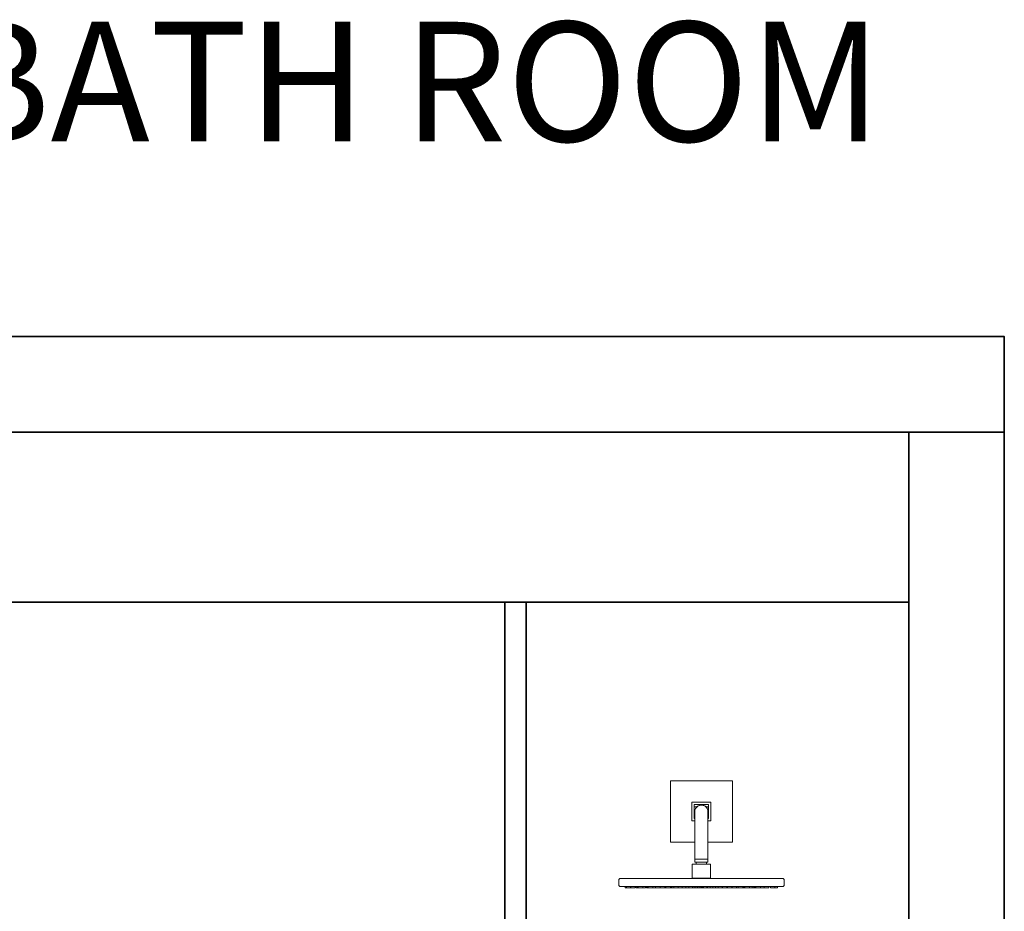
# Model space of a CAD drawing. Units: inches. Extents: x 64 to 1167, y 117 to 939.
# Tile 56 of 56: x 1074 to 1167, y 512 to 596. Entities that reach past the tile are written whole.
import ezdxf

# ---------------------------------------------------------------- set-up
doc = ezdxf.new("R2010")
doc.units = ezdxf.units.IN
doc.header["$MEASUREMENT"] = 0
for name, color, linetype, lineweight in [('A-ANNO-TEXT', 7, 'Continuous', 25), ('A-FLOR-FIXT', 8, 'Continuous', 18), ('A-SECT', 7, 'Continuous', 35)]:
    doc.layers.add(name, color=color, linetype=linetype, lineweight=lineweight)
doc.styles.get("Standard").update_dxf_attribs({"font": 'arial.ttf'})

msp = doc.modelspace()

# ---------------------------------------------------------------- linework, layer by layer
at = {"layer": 'A-FLOR-FIXT'}
for p, q in [((1141.249, 523.875), (1135.4, 523.875)), ((1135.4, 518.097), (1135.4, 523.875)), ((1141.249, 518.097), (1141.249, 523.875)), ((1137.42, 520.097), (1137.42, 521.875)), ((1137.429, 521.875), (1137.42, 521.875)), ((1137.438, 521.875), (1137.429, 521.875)), ((1137.447, 521.875), (1137.438, 521.875)), ((1137.455, 521.875), (1137.447, 521.875)), ((1137.462, 521.875), (1137.455, 521.875)), ((1137.468, 521.875), (1137.462, 521.875)), ((1137.473, 521.875), (1137.468, 521.875)), ((1137.477, 521.875), (1137.473, 521.875)), ((1137.48, 521.875), (1137.477, 521.875)), ((1137.482, 521.875), (1137.48, 521.875)), ((1137.48, 521.875), (1137.483, 521.875)), ((1139.148, 521.875), (1137.483, 521.875)), ((1139.15, 521.875), (1139.148, 521.875)), ((1139.153, 521.875), (1139.15, 521.875)), ((1139.157, 521.875), (1139.153, 521.875)), ((1139.162, 521.875), (1139.157, 521.875)), ((1139.169, 521.875), (1139.162, 521.875)), ((1139.176, 521.875), (1139.169, 521.875)), ((1139.184, 521.875), (1139.176, 521.875)), ((1139.192, 521.875), (1139.184, 521.875)), ((1139.201, 521.875), (1139.192, 521.875)), ((1139.21, 521.875), (1139.201, 521.875)), ((1139.21, 520.097), (1139.21, 521.875)), ((1137.641, 521.43), (1137.641, 521.653)), ((1137.641, 521.653), (1138.991, 521.653)), ((1137.882, 521.43), (1137.641, 521.43)), ((1137.641, 520.319), (1137.641, 521.43)), ((1137.681, 520.967), (1137.702, 521.128)), ((1137.702, 520.806), (1137.681, 520.967)), ((1137.681, 520.319), (1137.681, 520.967)), ((1137.694, 520.986), (1137.702, 521.054)), ((1137.702, 520.918), (1137.694, 520.986)), ((1137.702, 521.128), (1137.765, 521.278)), ((1137.765, 521.278), (1137.774, 521.291)), ((1137.774, 521.291), (1137.777, 521.297)), ((1137.777, 521.297), (1137.864, 521.407)), ((1137.864, 521.407), (1137.894, 521.43)), ((1137.864, 521.407), (1137.876, 521.426)), ((1137.876, 521.426), (1137.882, 521.43)), ((1137.882, 521.43), (1138.005, 521.525)), ((1137.894, 521.43), (1137.882, 521.43)), ((1137.894, 521.43), (1137.992, 521.506)), ((1137.992, 521.506), (1138.142, 521.568)), ((1138.005, 521.525), (1138.155, 521.587)), ((1138.142, 521.568), (1138.303, 521.589)), ((1138.155, 521.587), (1138.316, 521.608)), ((1138.303, 521.589), (1138.464, 521.568)), ((1138.316, 521.608), (1138.477, 521.587)), ((1138.464, 521.568), (1138.615, 521.506)), ((1138.477, 521.587), (1138.627, 521.525)), ((1138.615, 521.506), (1138.713, 521.43)), ((1138.627, 521.525), (1138.75, 521.43)), ((1138.75, 521.43), (1138.713, 521.43)), ((1138.713, 521.43), (1138.743, 521.407)), ((1138.743, 521.407), (1138.842, 521.278)), ((1138.991, 521.43), (1138.75, 521.43)), ((1138.75, 521.43), (1138.756, 521.426)), ((1138.756, 521.426), (1138.855, 521.297)), ((1138.842, 521.278), (1138.904, 521.128)), ((1138.855, 521.297), (1138.917, 521.147)), ((1138.904, 521.128), (1138.926, 520.967)), ((1138.917, 521.147), (1138.938, 520.986)), ((1138.938, 520.986), (1138.926, 520.893)), ((1138.926, 520.893), (1138.926, 520.967)), ((1138.926, 520.319), (1138.926, 520.893)), ((1138.991, 521.43), (1138.991, 521.653)), ((1138.991, 520.319), (1138.991, 521.43)), ((1137.429, 520.097), (1137.42, 520.097)), ((1137.438, 520.097), (1137.429, 520.097)), ((1137.447, 520.097), (1137.438, 520.097)), ((1137.455, 520.097), (1137.447, 520.097)), ((1137.462, 520.097), (1137.455, 520.097)), ((1137.468, 520.097), (1137.462, 520.097)), ((1137.473, 520.097), (1137.468, 520.097)), ((1137.477, 520.097), (1137.473, 520.097)), ((1137.48, 520.097), (1137.477, 520.097)), ((1137.482, 520.097), (1137.48, 520.097)), ((1137.482, 520.097), (1137.483, 520.097)), ((1137.483, 520.097), (1137.681, 520.097)), ((1137.641, 520.319), (1137.681, 520.319)), ((1137.681, 520.097), (1137.681, 520.319)), ((1137.681, 518.097), (1137.681, 520.097)), ((1138.926, 520.319), (1138.991, 520.319)), ((1138.926, 520.097), (1138.926, 520.319)), ((1138.926, 520.097), (1139.148, 520.097)), ((1138.926, 518.097), (1138.926, 520.097)), ((1139.15, 520.097), (1139.148, 520.097)), ((1139.153, 520.097), (1139.15, 520.097)), ((1139.157, 520.097), (1139.153, 520.097)), ((1139.162, 520.097), (1139.157, 520.097)), ((1139.169, 520.097), (1139.162, 520.097)), ((1139.176, 520.097), (1139.169, 520.097)), ((1139.184, 520.097), (1139.176, 520.097)), ((1139.192, 520.097), (1139.184, 520.097)), ((1139.201, 520.097), (1139.192, 520.097)), ((1139.21, 520.097), (1139.201, 520.097)), ((1135.4, 518.097), (1137.681, 518.097)), ((1137.681, 518.097), (1137.702, 518.097)), ((1137.681, 516.515), (1137.681, 518.097)), ((1138.926, 518.097), (1141.249, 518.097)), ((1138.926, 516.515), (1138.926, 518.097)), ((1137.681, 516.204), (1137.681, 516.515)), ((1138.926, 516.515), (1137.681, 516.515)), ((1137.828, 516.204), (1137.681, 516.204)), ((1137.828, 516.204), (1137.828, 516.035)), ((1138.779, 516.204), (1137.828, 516.204)), ((1138.779, 516.204), (1138.779, 516.035)), ((1138.926, 516.204), (1138.779, 516.204)), ((1138.926, 516.204), (1138.926, 516.515)), ((1137.442, 516.035), (1137.442, 514.726)), ((1137.442, 516.035), (1137.828, 516.035)), ((1137.828, 516.035), (1138.779, 516.035)), ((1138.779, 516.035), (1139.165, 516.035)), ((1139.165, 516.035), (1139.165, 514.726)), ((1130.617, 514.681), (1130.528, 514.592)), ((1130.528, 514.592), (1130.528, 514.015)), ((1130.617, 514.681), (1137.668, 514.681)), ((1137.442, 514.726), (1137.668, 514.726)), ((1137.668, 514.726), (1137.668, 514.681)), ((1138.939, 514.726), (1137.668, 514.726)), ((1137.668, 514.681), (1138.939, 514.681)), ((1138.939, 514.726), (1138.939, 514.681)), ((1138.939, 514.726), (1139.165, 514.726)), ((1145.992, 514.681), (1138.939, 514.681)), ((1145.992, 514.681), (1146.081, 514.592)), ((1146.081, 514.592), (1146.081, 514.015)), ((1130.617, 513.926), (1130.528, 514.015)), ((1131.125, 513.926), (1130.617, 513.926)), ((1131.125, 513.926), (1131.125, 513.793)), ((1131.262, 513.926), (1131.125, 513.926)), ((1131.125, 513.793), (1131.262, 513.793)), ((1131.262, 513.926), (1131.262, 513.793)), ((1131.262, 513.926), (1131.622, 513.926)), ((1131.262, 513.793), (1131.622, 513.793)), ((1131.622, 513.926), (1131.632, 513.926)), ((1131.622, 513.926), (1131.622, 513.793)), ((1131.632, 513.926), (1131.674, 513.926)), ((1131.632, 513.926), (1131.632, 513.793)), ((1131.632, 513.793), (1131.674, 513.793)), ((1131.674, 513.926), (1131.674, 513.793)), ((1131.674, 513.926), (1132.079, 513.926)), ((1131.674, 513.793), (1132.079, 513.793)), ((1132.079, 513.926), (1132.079, 513.793)), ((1132.162, 513.926), (1132.079, 513.926)), ((1132.162, 513.926), (1132.279, 513.926)), ((1132.162, 513.926), (1132.162, 513.793)), ((1132.279, 513.793), (1132.162, 513.793)), ((1132.279, 513.926), (1132.279, 513.793)), ((1132.279, 513.926), (1132.357, 513.926)), ((1132.357, 513.793), (1132.279, 513.793)), ((1132.357, 513.926), (1132.357, 513.793)), ((1132.357, 513.926), (1132.791, 513.926)), ((1132.357, 513.793), (1132.791, 513.793)), ((1132.791, 513.926), (1132.791, 513.793)), ((1133.032, 513.926), (1132.791, 513.926)), ((1133.032, 513.793), (1132.791, 513.793)), ((1133.032, 513.926), (1133.154, 513.926)), ((1133.032, 513.926), (1133.032, 513.793)), ((1133.154, 513.926), (1133.199, 513.926)), ((1133.154, 513.926), (1133.154, 513.793)), ((1133.154, 513.793), (1133.199, 513.793)), ((1133.199, 513.926), (1133.209, 513.926)), ((1133.199, 513.926), (1133.199, 513.793)), ((1133.199, 513.793), (1133.209, 513.793)), ((1133.209, 513.926), (1133.285, 513.926)), ((1133.209, 513.926), (1133.209, 513.793)), ((1133.285, 513.793), (1133.209, 513.793)), ((1133.285, 513.926), (1133.285, 513.793)), ((1133.285, 513.926), (1133.729, 513.926)), ((1133.285, 513.793), (1133.729, 513.793)), ((1133.729, 513.926), (1133.986, 513.926)), ((1133.729, 513.926), (1133.729, 513.793)), ((1133.986, 513.793), (1133.729, 513.793)), ((1133.986, 513.926), (1134, 513.926)), ((1133.986, 513.926), (1133.986, 513.793)), ((1133.986, 513.793), (1134, 513.793)), ((1134, 513.926), (1134, 513.793)), ((1134, 513.926), (1134.418, 513.926)), ((1134, 513.793), (1134.418, 513.793)), ((1134.418, 513.926), (1134.418, 513.793)), ((1134.418, 513.926), (1134.855, 513.926)), ((1134.418, 513.793), (1134.855, 513.793)), ((1134.855, 513.926), (1134.855, 513.793)), ((1134.855, 513.926), (1134.968, 513.926)), ((1134.968, 513.793), (1134.855, 513.793)), ((1134.968, 513.926), (1134.968, 513.793)), ((1134.968, 513.926), (1135.405, 513.926)), ((1135.405, 513.793), (1134.968, 513.793)), ((1135.405, 513.926), (1135.431, 513.926)), ((1135.405, 513.926), (1135.405, 513.793)), ((1135.405, 513.793), (1135.431, 513.793)), ((1135.431, 513.926), (1135.517, 513.926)), ((1135.431, 513.926), (1135.431, 513.793)), ((1135.517, 513.793), (1135.431, 513.793)), ((1135.517, 513.926), (1135.711, 513.926)), ((1135.517, 513.926), (1135.517, 513.793)), ((1135.517, 513.793), (1135.711, 513.793)), ((1135.711, 513.926), (1135.711, 513.793)), ((1135.711, 513.926), (1136.123, 513.926)), ((1135.711, 513.793), (1136.123, 513.793)), ((1136.123, 513.926), (1136.123, 513.793)), ((1136.484, 513.926), (1136.123, 513.926)), ((1136.123, 513.793), (1136.484, 513.793)), ((1136.484, 513.926), (1136.484, 513.793)), ((1136.484, 513.926), (1136.845, 513.926)), ((1136.484, 513.793), (1136.618, 513.793)), ((1136.616, 513.793), (1136.618, 513.793)), ((1136.845, 513.793), (1136.618, 513.793)), ((1136.845, 513.926), (1136.845, 513.793)), ((1136.845, 513.926), (1137.11, 513.926)), ((1137.11, 513.793), (1136.845, 513.793)), ((1137.11, 513.926), (1137.11, 513.793)), ((1137.48, 513.926), (1137.11, 513.926)), ((1137.11, 513.793), (1137.48, 513.793)), ((1137.48, 513.926), (1137.48, 513.793)), ((1137.48, 513.926), (1137.638, 513.926)), ((1137.48, 513.793), (1137.638, 513.793)), ((1137.638, 513.926), (1137.638, 513.793)), ((1137.638, 513.926), (1137.795, 513.926)), ((1137.795, 513.793), (1137.638, 513.793)), ((1137.795, 513.926), (1137.795, 513.793)), ((1137.795, 513.926), (1137.953, 513.926)), ((1137.953, 513.793), (1137.795, 513.793)), ((1137.953, 513.926), (1137.953, 513.793)), ((1137.953, 513.926), (1138.111, 513.926)), ((1138.111, 513.793), (1137.953, 513.793)), ((1138.111, 513.926), (1138.111, 513.793)), ((1138.269, 513.926), (1138.111, 513.926)), ((1138.269, 513.793), (1138.111, 513.793)), ((1138.269, 513.926), (1138.285, 513.926)), ((1138.269, 513.926), (1138.269, 513.793)), ((1138.269, 513.793), (1138.285, 513.793)), ((1138.285, 513.926), (1138.331, 513.926)), ((1138.285, 513.926), (1138.285, 513.793)), ((1138.285, 513.793), (1138.331, 513.793)), ((1138.331, 513.926), (1138.376, 513.926)), ((1138.331, 513.926), (1138.331, 513.793)), ((1138.376, 513.793), (1138.331, 513.793)), ((1138.376, 513.926), (1138.421, 513.926)), ((1138.376, 513.926), (1138.376, 513.793)), ((1138.421, 513.793), (1138.376, 513.793)), ((1138.421, 513.926), (1138.466, 513.926)), ((1138.421, 513.926), (1138.421, 513.793)), ((1138.466, 513.793), (1138.421, 513.793)), ((1138.466, 513.926), (1138.512, 513.926)), ((1138.466, 513.926), (1138.466, 513.793)), ((1138.466, 513.793), (1138.512, 513.793)), ((1138.512, 513.926), (1138.826, 513.926)), ((1138.512, 513.926), (1138.512, 513.793)), ((1138.826, 513.793), (1138.512, 513.793)), ((1138.826, 513.926), (1138.826, 513.793)), ((1138.826, 513.926), (1138.875, 513.926)), ((1138.875, 513.793), (1138.826, 513.793)), ((1138.875, 513.926), (1138.875, 513.793)), ((1139.128, 513.926), (1138.875, 513.926)), ((1138.875, 513.793), (1139.128, 513.793)), ((1139.128, 513.926), (1139.128, 513.793)), ((1139.128, 513.926), (1139.381, 513.926)), ((1139.381, 513.793), (1139.128, 513.793)), ((1139.381, 513.926), (1139.381, 513.793)), ((1139.634, 513.926), (1139.381, 513.926)), ((1139.634, 513.793), (1139.381, 513.793)), ((1139.634, 513.926), (1139.634, 513.793)), ((1139.887, 513.926), (1139.634, 513.926)), ((1139.634, 513.793), (1139.887, 513.793)), ((1139.887, 513.926), (1139.887, 513.793)), ((1139.887, 513.926), (1140.258, 513.926)), ((1140.258, 513.793), (1139.887, 513.793)), ((1140.258, 513.926), (1140.258, 513.793)), ((1140.258, 513.926), (1140.297, 513.926)), ((1140.258, 513.793), (1140.297, 513.793)), ((1140.297, 513.926), (1140.297, 513.793)), ((1140.71, 513.926), (1140.297, 513.926)), ((1140.71, 513.793), (1140.297, 513.793)), ((1140.71, 513.926), (1140.71, 513.793)), ((1140.71, 513.926), (1140.748, 513.926)), ((1140.71, 513.793), (1140.748, 513.793)), ((1140.748, 513.926), (1140.748, 513.793)), ((1140.748, 513.926), (1141.16, 513.926)), ((1141.16, 513.793), (1140.748, 513.793)), ((1141.16, 513.926), (1141.16, 513.793)), ((1141.16, 513.926), (1141.198, 513.926)), ((1141.16, 513.793), (1141.198, 513.793)), ((1141.198, 513.926), (1141.198, 513.793)), ((1141.611, 513.926), (1141.198, 513.926)), ((1141.611, 513.793), (1141.198, 513.793)), ((1141.611, 513.926), (1141.611, 513.793)), ((1141.611, 513.926), (1141.761, 513.926)), ((1141.761, 513.793), (1141.611, 513.793)), ((1141.761, 513.926), (1141.761, 513.793)), ((1141.761, 513.926), (1142.198, 513.926)), ((1142.198, 513.793), (1141.761, 513.793)), ((1142.198, 513.926), (1142.198, 513.793)), ((1142.198, 513.926), (1142.294, 513.926)), ((1142.294, 513.793), (1142.198, 513.793)), ((1142.294, 513.926), (1142.294, 513.793)), ((1142.371, 513.926), (1142.294, 513.926)), ((1142.371, 513.793), (1142.294, 513.793)), ((1142.371, 513.926), (1142.371, 513.793)), ((1142.371, 513.926), (1142.39, 513.926)), ((1142.371, 513.793), (1142.39, 513.793)), ((1142.39, 513.926), (1142.39, 513.793)), ((1142.828, 513.926), (1142.39, 513.926)), ((1142.828, 513.793), (1142.39, 513.793)), ((1142.828, 513.926), (1142.828, 513.793)), ((1142.828, 513.926), (1143.076, 513.926)), ((1143.076, 513.793), (1142.828, 513.793)), ((1143.076, 513.926), (1143.076, 513.793)), ((1143.229, 513.926), (1143.076, 513.926)), ((1143.229, 513.793), (1143.076, 513.793)), ((1143.229, 513.926), (1143.229, 513.793)), ((1143.229, 513.926), (1143.326, 513.926)), ((1143.326, 513.793), (1143.229, 513.793)), ((1143.326, 513.926), (1143.415, 513.926)), ((1143.326, 513.926), (1143.326, 513.793)), ((1143.415, 513.793), (1143.326, 513.793)), ((1143.415, 513.926), (1143.415, 513.793)), ((1143.415, 513.926), (1143.859, 513.926)), ((1143.859, 513.793), (1143.415, 513.793)), ((1143.859, 513.926), (1143.859, 513.793)), ((1144.217, 513.926), (1143.859, 513.926)), ((1144.217, 513.793), (1143.859, 513.793)), ((1144.217, 513.926), (1144.217, 513.793)), ((1144.217, 513.926), (1144.229, 513.926)), ((1144.217, 513.793), (1144.229, 513.793)), ((1144.229, 513.926), (1144.229, 513.793)), ((1144.662, 513.926), (1144.229, 513.926)), ((1144.662, 513.793), (1144.229, 513.793)), ((1144.662, 513.926), (1144.799, 513.926)), ((1144.662, 513.926), (1144.662, 513.793)), ((1144.799, 513.926), (1144.801, 513.926)), ((1144.799, 513.926), (1144.799, 513.793)), ((1144.799, 513.793), (1144.801, 513.793)), ((1144.801, 513.926), (1144.801, 513.793)), ((1145.205, 513.926), (1144.801, 513.926)), ((1145.205, 513.793), (1144.801, 513.793)), ((1145.205, 513.926), (1145.205, 513.793)), ((1145.464, 513.926), (1145.205, 513.926)), ((1145.464, 513.793), (1145.205, 513.793)), ((1145.464, 513.926), (1145.464, 513.793)), ((1145.464, 513.926), (1145.992, 513.926)), ((1146.081, 514.015), (1145.992, 513.926))]:
    msp.add_line(p, q, dxfattribs=at)
at = {"layer": 'A-SECT'}
for p, q in [((1166.813, 556.679), (982.813, 556.679)), ((1157.813, 436.679), (1157.813, 556.679)), ((1157.813, 540.679), (991.813, 540.679)), ((1119.813, 436.679), (1119.813, 540.679)), ((1121.813, 436.679), (1121.813, 540.679))]:
    msp.add_line(p, q, dxfattribs=at)
msp.add_lwpolyline([(982.813, 427.679), (1166.813, 427.679), (1166.813, 565.679), (982.813, 565.679)], close=True, dxfattribs=at)

# ---------------------------------------------------------------- texts
at = {"layer": 'A-ANNO-TEXT'}
msp.add_text('SECTION OF BATH ROOM', height=11.26378, dxfattribs=at).set_placement((975.962, 584.046))

doc.saveas('drawing.dxf')
